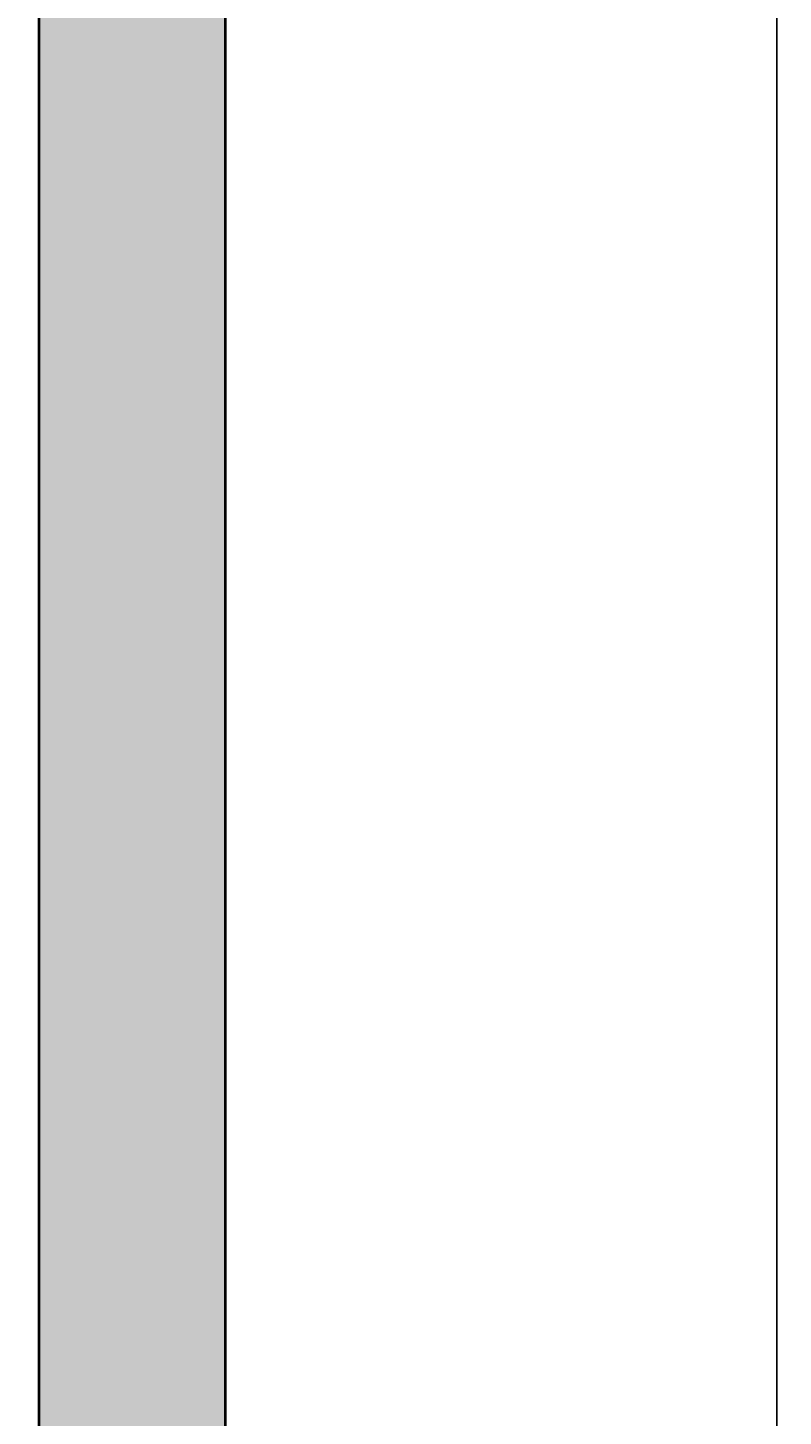
# Model space of a CAD drawing. Units: inches. Extents: x 1441 to 2460, y 1648 to 2683.
# Tile 9 of 35: x 1880 to 1916, y 1866 to 1933. Entities that reach past the tile are written whole.
import ezdxf

# ---------------------------------------------------------------- set-up
doc = ezdxf.new("R2010")
doc.units = ezdxf.units.IN
doc.layers.add('A-ANNO-DIMS', color=2, linetype='Continuous', lineweight=18)
doc.layers.add('A-WALL', color=7, linetype='Continuous', lineweight=40)
doc.layers.add('A-WALL-PATT', color=251, linetype='Continuous', lineweight=13, true_color=0x636466)
doc.styles.get("Standard").update_dxf_attribs({"font": 'arial.ttf'})
doc.dimstyles.get("Standard").update_dxf_attribs({"dimtxt": 0.18, "dimasz": 0.18, "dimexe": 0.18, "dimexo": 0.0625, "dimgap": 0.09, "dimtad": 0, "dimtih": 1, "dimtoh": 1, "dimdec": 4, "dimzin": 0, "dimdsep": 46, "dimtxsty": 'Standard', "dimcen": 0.09, "dimadec": 0, "dimazin": 0, "dimtfac": 1, "dimtdec": 4, "dimtofl": 0, "dimtmove": 0, "dimatfit": 3, "dimfxl": 1, "dimtolj": 1, "dimtzin": 0, "dimarcsym": 0})

# ---------------------------------------------------------------- blocks, each defined once
blk = doc.blocks.new('*D67')
at = {"layer": 'A-ANNO-DIMS', "color": 0, "lineweight": -2, "transparency": 16777216}
for p, q in [((1889.448, 2298.695), (1916.216, 2298.695)), ((1916.036, 2298.515), (1916.036, 2055.938)), ((1916.036, 1812.997), (1916.036, 2055.574)), ((1758.224, 1812.817), (1916.216, 1812.817))]:
    blk.add_line(p, q, dxfattribs=at)
at = {"layer": 'A-ANNO-DIMS', "color": 0, "transparency": 16777216}
for points in [[(1916.006, 2298.515), (1916.066, 2298.515), (1916.036, 2298.695)], [(1916.006, 1812.997), (1916.066, 1812.997), (1916.036, 1812.817)]]:
    blk.add_solid(points, dxfattribs=at)
at = {"layer": 'Defpoints', "color": 0, "transparency": 16777216}
for p in [(1889.386, 2298.695), (1916.036, 2298.695), (1758.161, 1812.817)]:
    blk.add_point(p, dxfattribs=at)
at = {"layer": 'A-ANNO-DIMS', "color": 0, "transparency": 16777216, "insert": (1916.036, 2055.756), "char_height": 0.18, "attachment_point": 5}
blk.add_mtext('\\A1;485.9', dxfattribs=at)

msp = doc.modelspace()

# ---------------------------------------------------------------- hatches: boundary and pattern name
at = {"layer": 'A-WALL-PATT'}
h = msp.add_hatch(color=256, dxfattribs=at)
h.dxf.hatch_style = 1
h.paths.add_polyline_path([(1627.5085, 2298.6952), (1568.8859, 2298.6952), (1568.8859, 2246.9605), (1577.8859, 2246.9605), (1577.8859, 2289.6952), (1627.5085, 2289.6952), (1627.5085, 2294.1952)])
h.paths.add_polyline_path([(1675.5777, 2298.6952), (1651.5085, 2298.6952), (1651.5085, 2289.6952), (1675.5777, 2289.6952), (1675.5777, 2294.1952)])
h.paths.add_polyline_path([(1667.3859, 2289.6952), (1662.8859, 2289.6952), (1662.8859, 2233.0622), (1667.3859, 2233.0622)])
h.paths.add_polyline_path([(1715.8721, 2294.3362), (1715.8721, 2295.2788), (1715.8721, 2298.6952), (1699.5777, 2298.6952), (1699.5777, 2289.6952), (1715.8721, 2289.6952)])
h.paths.add_polyline_path([(1707.8859, 2289.6952), (1703.3859, 2289.6952), (1703.3859, 2199.6952), (1707.8859, 2199.6952)])
h.paths.add_polyline_path([(1760.3859, 2204.637), (1755.8859, 2204.637), (1755.8859, 2199.6952), (1667.3859, 2199.6952), (1667.3859, 2204.637), (1662.8859, 2204.637), (1662.8859, 2195.1952), (1760.3859, 2195.1952)])
h.paths.add_polyline_path([(1760.3859, 2289.6952), (1755.8859, 2289.6952), (1755.8859, 2233.0622), (1760.3859, 2233.0622)])
h.paths.add_polyline_path([(1889.3859, 2298.6952), (1739.8721, 2298.6952), (1739.8721, 2289.6952), (1880.3859, 2289.6952), (1880.3859, 2250.8051), (1889.3859, 2250.8051)])
h.paths.add_polyline_path([(1889.3859, 2202.8051), (1880.3859, 2202.8051), (1880.3859, 2157.6952), (1747.948, 2157.6952), (1747.948, 2153.1952), (1755.8859, 2153.1952), (1755.8859, 2058.005), (1760.3859, 2058.005), (1760.3859, 2153.1952), (1880.3859, 2153.1952), (1880.3859, 2124.108), (1889.3859, 2124.108)])
h.paths.add_polyline_path([(1889.3859, 1984.8305), (1880.3859, 1984.8305), (1880.3859, 1834.1952), (1889.3859, 1834.1952)])
h.paths.add_polyline_path([(1889.3859, 2076.108), (1880.3859, 2076.108), (1880.3859, 2008.8305), (1889.3859, 2008.8305)])
h.paths.add_polyline_path([(1880.3859, 2027.1952), (1800.8859, 2027.1952), (1800.8859, 2000.9452), (1805.3859, 2000.9452), (1805.3859, 2022.6952), (1880.3859, 2022.6952)])
h.paths.add_polyline_path([(1800.8859, 2027.1952), (1760.3859, 2027.1952), (1760.3859, 2030.7912), (1755.8859, 2030.7912), (1755.8859, 2022.6952), (1800.8859, 2022.6952)])
h.paths.add_polyline_path([(1880.3859, 1974.6952), (1805.3859, 1974.6952), (1805.3859, 1978.7973), (1800.8859, 1978.7973), (1800.8859, 1974.6952), (1794.8823, 1974.6952), (1794.8823, 1970.1952), (1800.8859, 1970.1952), (1805.3859, 1970.1952), (1880.3859, 1970.1952)])
h.paths.add_polyline_path([(1760.3859, 1974.6952), (1755.8859, 1974.6952), (1755.8859, 1925.6952), (1751.8616, 1925.6952), (1751.8616, 1921.1952), (1760.3859, 1921.1952)])
h.paths.add_polyline_path([(1760.3859, 1921.1952), (1755.8859, 1921.1952), (1755.8859, 1843.1952), (1760.3859, 1843.1952)])
h.paths.add_polyline_path([(1799.1136, 1838.6952), (1799.1136, 1843.1952), (1760.3859, 1843.1952), (1751.8944, 1843.1952), (1751.8944, 1834.1952), (1758.1615, 1834.1952), (1799.1136, 1834.1952)])
h.paths.add_polyline_path([(1880.3859, 1843.1952), (1859.1136, 1843.1952), (1859.1136, 1834.1952), (1880.3859, 1834.1952)])
h.paths.add_polyline_path([(1577.8859, 1857.7914), (1568.8859, 1857.7914), (1568.8859, 1834.1952), (1695.0034, 1834.1952), (1695.0034, 1838.6952), (1695.0034, 1843.1952), (1577.8859, 1843.1952)])
h.paths.add_polyline_path([(1577.8859, 1959.2399), (1573.3859, 1959.2399), (1568.8859, 1959.2399), (1568.8859, 1905.7914), (1577.8859, 1905.7914), (1577.8859, 1921.1952), (1703.3859, 1921.1952), (1707.8859, 1921.1952), (1715.1501, 1921.1952), (1715.1501, 1925.6952), (1707.8859, 1925.6952), (1703.3859, 1925.6952), (1577.8859, 1925.6952)])
h.paths.add_polyline_path([(1577.8859, 2106.6907), (1568.8859, 2106.6907), (1568.8859, 2019.2399), (1577.8859, 2019.2399)])
h.paths.add_polyline_path([(1707.8859, 2051.6952), (1703.3859, 2051.6952), (1703.3859, 2048.6952), (1703.3859, 1925.6952), (1707.8859, 1925.6952)])
h.paths.add_polyline_path([(1703.3859, 2051.6952), (1676.3859, 2051.6952), (1676.3859, 2048.6952), (1703.3859, 2048.6952)])
h.paths.add_polyline_path([(1703.3859, 2102.6952), (1676.3859, 2102.6952), (1676.3859, 2099.6952), (1685.3859, 2099.6952), (1703.3859, 2099.6952)])
h.paths.add_polyline_path([(1707.8859, 2153.1952), (1710.5611, 2153.1952), (1710.5611, 2157.6952), (1707.8859, 2157.6952), (1707.8859, 2195.1952), (1703.3859, 2195.1952), (1703.3859, 2099.6952), (1707.8859, 2099.6952)])
h.paths.add_polyline_path([(1577.8859, 2198.9605), (1568.8859, 2198.9605), (1568.8859, 2166.6907), (1577.8859, 2166.6907)])

# ---------------------------------------------------------------- linework, layer by layer
at = {"layer": 'A-WALL'}
for p, q in [((1889.3859, 2298.6952), (1889.3859, 1834.1952)), ((1880.3859, 2153.1952), (1880.3859, 1834.1952))]:
    msp.add_line(p, q, dxfattribs=at)

# ---------------------------------------------------------------- dimensions: what is measured, and where the dimension line sits
at = {"layer": 'A-ANNO-DIMS'}
dim = msp.add_linear_dim(base=(1916.0359, 2298.6952), p1=(1758.1615, 1812.8171), p2=(1889.3859, 2298.6952), angle=90, dimstyle='Standard', override={"dimdec": 1, "dimlfac": 1, "dimrnd": 0, "dimzin": 0, "dimdsep": 46, "dimlunit": 2}, dxfattribs=at)
dim.commit()
dim.dimension.update_dxf_attribs({"geometry": '*D67', "text_midpoint": (1916.0359, 2055.7561)})

doc.saveas('drawing.dxf')
